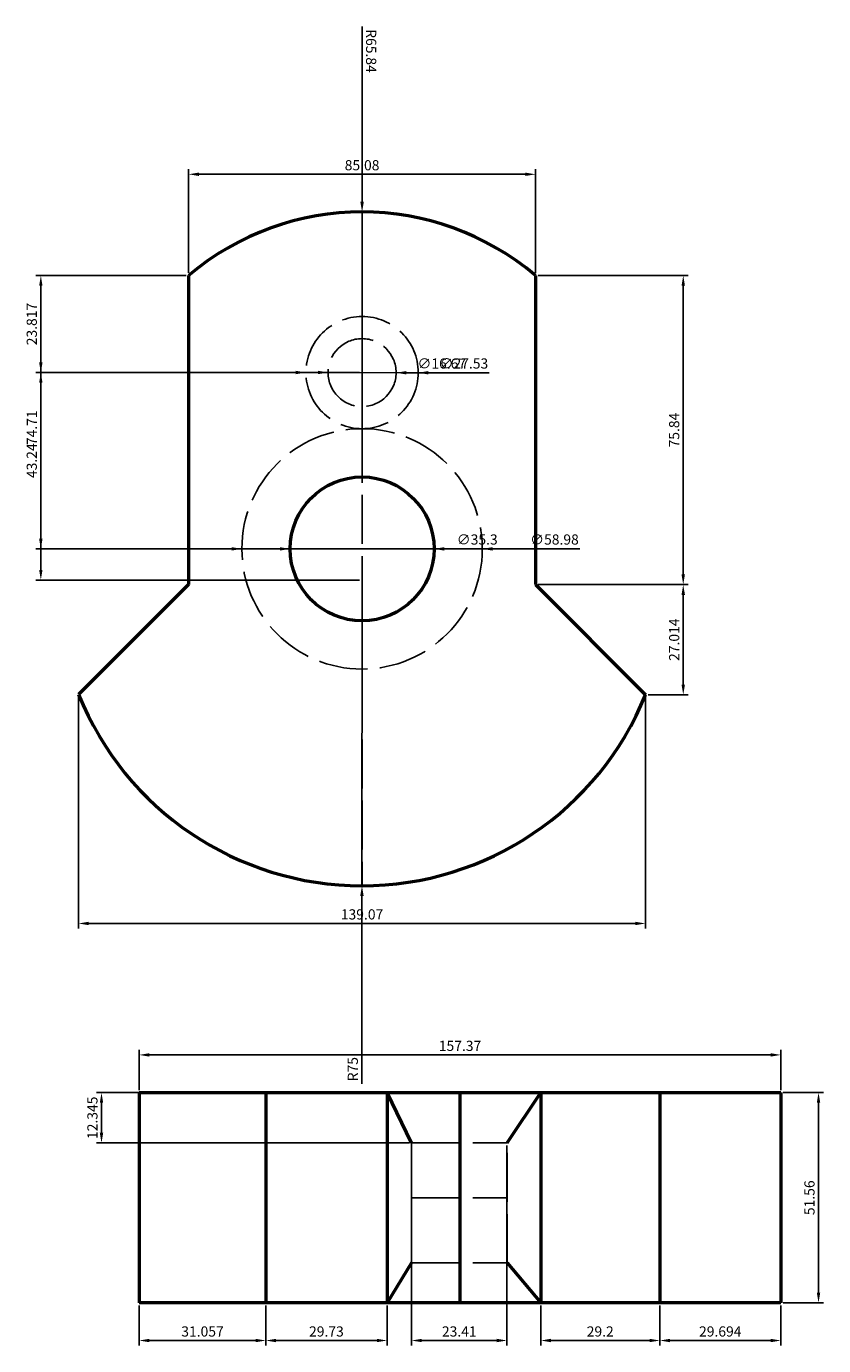
# Model space of a CAD drawing. Units: millimetres. Extents: x 921 to 2648, y 1390 to 2315.
# Tile 5 of 10: x 1425 to 1621, y 1915 to 2239. Entities that reach past the tile are written whole.
import ezdxf

# ---------------------------------------------------------------- set-up
doc = ezdxf.new("R2010")
doc.units = ezdxf.units.MM
doc.linetypes.add('ACAD_ISO02W100', pattern=[15, 12, -3])
for name, color, linetype, lineweight in [('M-DIMS', 2, 'Continuous', 25), ('M-HIDN', 4, 'ACAD_ISO02W100', 25), ('M-OUTL', 7, 'Continuous', 50)]:
    doc.layers.add(name, color=color, linetype=linetype, lineweight=lineweight)
doc.styles.get("Standard").update_dxf_attribs({"font": 'arial.ttf'})
doc.dimstyles.new('ISO-25', dxfattribs={"dimtxt": 2.5, "dimasz": 2.5, "dimexe": 1.25, "dimexo": 0.625, "dimtad": 1, "dimtxsty": 'Standard', "dimcen": 2.5, "dimadec": 0, "dimazin": 0, "dimtfac": 1, "dimtmove": 0, "dimatfit": 3, "dimfxl": 1, "dimarcsym": 0})

# ---------------------------------------------------------------- blocks, each defined once
blk = doc.blocks.new('*D26')
at = {"layer": 'Defpoints', "color": 0, "transparency": 16777216}
for p in [(1550.34, 2202.68), (1465.26, 2177.84), (1550.34, 2177.84)]:
    blk.add_point(p, dxfattribs=at)
at = {"layer": 'M-DIMS', "color": 0, "lineweight": -2, "transparency": 16777216}
for p, q in [((1465.26, 2178.47), (1465.26, 2203.93)), ((1467.76, 2202.68), (1547.84, 2202.68)), ((1550.34, 2178.47), (1550.34, 2203.93))]:
    blk.add_line(p, q, dxfattribs=at)
at = {"layer": 'M-DIMS', "color": 0, "transparency": 16777216}
for points in [[(1467.76, 2203.1), (1467.76, 2202.27), (1465.26, 2202.68)], [(1547.84, 2203.1), (1547.84, 2202.27), (1550.34, 2202.68)]]:
    blk.add_solid(points, dxfattribs=at)
at = {"layer": 'M-DIMS', "color": 0, "transparency": 16777216, "insert": (1507.8, 2204.58), "char_height": 2.5, "attachment_point": 5}
blk.add_mtext('85.08', dxfattribs=at)
blk = doc.blocks.new('*D27')
at = {"layer": 'Defpoints', "color": 0, "transparency": 16777216}
for p in [(1610.5, 1986.64), (1453.13, 1977.39), (1610.5, 1977.39)]:
    blk.add_point(p, dxfattribs=at)
at = {"layer": 'M-DIMS', "color": 0, "lineweight": -2, "transparency": 16777216}
for p, q in [((1453.13, 1978.01), (1453.13, 1987.89)), ((1610.5, 1978.01), (1610.5, 1987.89)), ((1455.63, 1986.64), (1608, 1986.64))]:
    blk.add_line(p, q, dxfattribs=at)
at = {"layer": 'M-DIMS', "color": 0, "transparency": 16777216}
for points in [[(1455.63, 1987.05), (1455.63, 1986.22), (1453.13, 1986.64)], [(1608, 1987.05), (1608, 1986.22), (1610.5, 1986.64)]]:
    blk.add_solid(points, dxfattribs=at)
at = {"layer": 'M-DIMS', "color": 0, "transparency": 16777216, "insert": (1531.82, 1988.54), "char_height": 2.5, "attachment_point": 5}
blk.add_mtext('157.37', dxfattribs=at)
blk = doc.blocks.new('*D28')
at = {"layer": 'Defpoints', "color": 0, "transparency": 16777216}
for p in [(1610.5, 1977.39), (1610.5, 1925.82), (1619.75, 1925.82)]:
    blk.add_point(p, dxfattribs=at)
at = {"layer": 'M-DIMS', "color": 0, "lineweight": -2, "transparency": 16777216}
for p, q in [((1611.12, 1977.39), (1621, 1977.39)), ((1619.75, 1974.89), (1619.75, 1928.32)), ((1611.12, 1925.82), (1621, 1925.82))]:
    blk.add_line(p, q, dxfattribs=at)
at = {"layer": 'M-DIMS', "color": 0, "transparency": 16777216}
for points in [[(1619.33, 1974.89), (1620.17, 1974.89), (1619.75, 1977.39)], [(1619.33, 1928.32), (1620.17, 1928.32), (1619.75, 1925.82)]]:
    blk.add_solid(points, dxfattribs=at)
at = {"layer": 'M-DIMS', "color": 0, "transparency": 16777216, "insert": (1617.85, 1951.6), "char_height": 2.5, "attachment_point": 5, "rotation": 90}
blk.add_mtext('51.56', dxfattribs=at)
blk = doc.blocks.new('*D62')
at = {"layer": 'Defpoints', "color": 0, "transparency": 16777216}
for p in [(1550.34, 2177.84), (1550.34, 2102.01), (1586.57, 2102.01)]:
    blk.add_point(p, dxfattribs=at)
at = {"layer": 'M-DIMS', "color": 0, "lineweight": -2, "transparency": 16777216}
for p, q in [((1550.96, 2177.84), (1587.82, 2177.84)), ((1586.57, 2175.34), (1586.57, 2104.51)), ((1550.96, 2102.01), (1587.82, 2102.01))]:
    blk.add_line(p, q, dxfattribs=at)
at = {"layer": 'M-DIMS', "color": 0, "transparency": 16777216}
for points in [[(1586.15, 2175.34), (1586.99, 2175.34), (1586.57, 2177.84)], [(1586.15, 2104.51), (1586.99, 2104.51), (1586.57, 2102.01)]]:
    blk.add_solid(points, dxfattribs=at)
at = {"layer": 'M-DIMS', "color": 0, "transparency": 16777216, "insert": (1584.67, 2139.93), "char_height": 2.5, "attachment_point": 5, "rotation": 90}
blk.add_mtext('75.84', dxfattribs=at)
blk = doc.blocks.new('*D63')
at = {"layer": 'Defpoints', "color": 0, "transparency": 16777216}
for p in [(1465.26, 2177.84), (1429.01, 2154.03), (1507.8, 2154.03)]:
    blk.add_point(p, dxfattribs=at)
at = {"layer": 'M-DIMS', "color": 0, "lineweight": -2, "transparency": 16777216}
for p, q in [((1464.64, 2177.84), (1427.76, 2177.84)), ((1429.01, 2175.34), (1429.01, 2156.53)), ((1507.18, 2154.03), (1427.76, 2154.03))]:
    blk.add_line(p, q, dxfattribs=at)
at = {"layer": 'M-DIMS', "color": 0, "transparency": 16777216}
for points in [[(1428.59, 2175.34), (1429.42, 2175.34), (1429.01, 2177.84)], [(1428.59, 2156.53), (1429.42, 2156.53), (1429.01, 2154.03)]]:
    blk.add_solid(points, dxfattribs=at)
at = {"layer": 'M-DIMS', "color": 0, "transparency": 16777216, "insert": (1427.1, 2165.94), "char_height": 2.5, "attachment_point": 5, "rotation": 90}
blk.add_mtext('23.817', dxfattribs=at)
blk = doc.blocks.new('*D64')
at = {"layer": 'Defpoints', "color": 0, "transparency": 16777216}
for p in [(1507.8, 2154.03), (1429.01, 2110.78), (1507.8, 2110.78)]:
    blk.add_point(p, dxfattribs=at)
at = {"layer": 'M-DIMS', "color": 0, "lineweight": -2, "transparency": 16777216}
for p, q in [((1507.18, 2154.03), (1427.76, 2154.03)), ((1429.01, 2151.53), (1429.01, 2113.28)), ((1507.18, 2110.78), (1427.76, 2110.78))]:
    blk.add_line(p, q, dxfattribs=at)
at = {"layer": 'M-DIMS', "color": 0, "transparency": 16777216}
for points in [[(1428.59, 2151.53), (1429.42, 2151.53), (1429.01, 2154.03)], [(1428.59, 2113.28), (1429.42, 2113.28), (1429.01, 2110.78)]]:
    blk.add_solid(points, dxfattribs=at)
at = {"layer": 'M-DIMS', "color": 0, "transparency": 16777216, "insert": (1427.1, 2132.41), "char_height": 2.5, "attachment_point": 5, "rotation": 90}
blk.add_mtext('43.24', dxfattribs=at)
blk = doc.blocks.new('*D65')
at = {"layer": 'Defpoints', "color": 0, "transparency": 16777216}
for p in [(1465.26, 2177.84), (1429.01, 2103.14), (1507.8, 2103.14)]:
    blk.add_point(p, dxfattribs=at)
at = {"layer": 'M-DIMS', "color": 0, "lineweight": -2, "transparency": 16777216}
for p, q in [((1464.64, 2177.84), (1427.76, 2177.84)), ((1429.01, 2175.34), (1429.01, 2105.64)), ((1507.18, 2103.14), (1427.76, 2103.14))]:
    blk.add_line(p, q, dxfattribs=at)
at = {"layer": 'M-DIMS', "color": 0, "transparency": 16777216}
for points in [[(1428.59, 2175.34), (1429.42, 2175.34), (1429.01, 2177.84)], [(1428.59, 2105.64), (1429.42, 2105.64), (1429.01, 2103.14)]]:
    blk.add_solid(points, dxfattribs=at)
at = {"layer": 'M-DIMS', "color": 0, "transparency": 16777216, "insert": (1427.13, 2140.49), "char_height": 2.5, "attachment_point": 5, "rotation": 90}
blk.add_mtext('74.71', dxfattribs=at)
blk = doc.blocks.new('*D66')
at = {"layer": 'Defpoints', "color": 0, "transparency": 16777216}
for p in [(1438.26, 2075.06), (1577.32, 2074.99), (1577.32, 2018.89)]:
    blk.add_point(p, dxfattribs=at)
at = {"layer": 'M-DIMS', "color": 0, "lineweight": -2, "transparency": 16777216}
for p, q in [((1438.26, 2074.43), (1438.26, 2017.64)), ((1577.32, 2074.37), (1577.32, 2017.64)), ((1440.76, 2018.89), (1574.82, 2018.89))]:
    blk.add_line(p, q, dxfattribs=at)
at = {"layer": 'M-DIMS', "color": 0, "transparency": 16777216}
for points in [[(1440.76, 2019.3), (1440.76, 2018.47), (1438.26, 2018.89)], [(1574.82, 2019.3), (1574.82, 2018.47), (1577.32, 2018.89)]]:
    blk.add_solid(points, dxfattribs=at)
at = {"layer": 'M-DIMS', "color": 0, "transparency": 16777216, "insert": (1507.79, 2020.79), "char_height": 2.5, "attachment_point": 5}
blk.add_mtext('139.07', dxfattribs=at)
blk = doc.blocks.new('*D67')
at = {"layer": 'Defpoints', "color": 0, "transparency": 16777216}
for p in [(1550.34, 2102.01), (1577.32, 2074.99), (1586.57, 2074.99)]:
    blk.add_point(p, dxfattribs=at)
at = {"layer": 'M-DIMS', "color": 0, "lineweight": -2, "transparency": 16777216}
for p, q in [((1550.96, 2102.01), (1587.82, 2102.01)), ((1586.57, 2099.51), (1586.57, 2077.49)), ((1577.95, 2074.99), (1587.82, 2074.99))]:
    blk.add_line(p, q, dxfattribs=at)
at = {"layer": 'M-DIMS', "color": 0, "transparency": 16777216}
for points in [[(1586.15, 2099.51), (1586.99, 2099.51), (1586.57, 2102.01)], [(1586.15, 2077.49), (1586.99, 2077.49), (1586.57, 2074.99)]]:
    blk.add_solid(points, dxfattribs=at)
at = {"layer": 'M-DIMS', "color": 0, "transparency": 16777216, "insert": (1584.67, 2088.5), "char_height": 2.5, "attachment_point": 5, "rotation": 90}
blk.add_mtext('27.014', dxfattribs=at)
blk = doc.blocks.new('*D68')
at = {"layer": 'Defpoints', "color": 0, "transparency": 16777216}
for p in [(1453.13, 1925.82), (1484.19, 1925.82), (1484.19, 1916.57)]:
    blk.add_point(p, dxfattribs=at)
at = {"layer": 'M-DIMS', "color": 0, "lineweight": -2, "transparency": 16777216}
for p, q in [((1453.13, 1925.2), (1453.13, 1915.32)), ((1484.19, 1925.2), (1484.19, 1915.32)), ((1455.63, 1916.57), (1481.69, 1916.57))]:
    blk.add_line(p, q, dxfattribs=at)
at = {"layer": 'M-DIMS', "color": 0, "transparency": 16777216}
for points in [[(1455.63, 1916.99), (1455.63, 1916.16), (1453.13, 1916.57)], [(1481.69, 1916.99), (1481.69, 1916.16), (1484.19, 1916.57)]]:
    blk.add_solid(points, dxfattribs=at)
at = {"layer": 'M-DIMS', "color": 0, "transparency": 16777216, "insert": (1468.66, 1918.47), "char_height": 2.5, "attachment_point": 5}
blk.add_mtext('31.057', dxfattribs=at)
blk = doc.blocks.new('*D69')
at = {"layer": 'Defpoints', "color": 0, "transparency": 16777216}
for p in [(1484.19, 1925.82), (1513.92, 1925.82), (1513.92, 1916.57)]:
    blk.add_point(p, dxfattribs=at)
at = {"layer": 'M-DIMS', "color": 0, "lineweight": -2, "transparency": 16777216}
for p, q in [((1484.19, 1925.2), (1484.19, 1915.32)), ((1513.92, 1925.2), (1513.92, 1915.32)), ((1486.69, 1916.57), (1511.42, 1916.57))]:
    blk.add_line(p, q, dxfattribs=at)
at = {"layer": 'M-DIMS', "color": 0, "transparency": 16777216}
for points in [[(1486.69, 1916.99), (1486.69, 1916.16), (1484.19, 1916.57)], [(1511.42, 1916.99), (1511.42, 1916.16), (1513.92, 1916.57)]]:
    blk.add_solid(points, dxfattribs=at)
at = {"layer": 'M-DIMS', "color": 0, "transparency": 16777216, "insert": (1499.05, 1918.47), "char_height": 2.5, "attachment_point": 5}
blk.add_mtext('29.73', dxfattribs=at)
blk = doc.blocks.new('*D70')
at = {"layer": 'Defpoints', "color": 0, "transparency": 16777216}
for p in [(1551.61, 1925.82), (1580.81, 1925.82), (1580.81, 1916.57)]:
    blk.add_point(p, dxfattribs=at)
at = {"layer": 'M-DIMS', "color": 0, "lineweight": -2, "transparency": 16777216}
for p, q in [((1551.61, 1925.2), (1551.61, 1915.32)), ((1580.81, 1925.2), (1580.81, 1915.32)), ((1554.11, 1916.57), (1578.31, 1916.57))]:
    blk.add_line(p, q, dxfattribs=at)
at = {"layer": 'M-DIMS', "color": 0, "transparency": 16777216}
for points in [[(1554.11, 1916.99), (1554.11, 1916.16), (1551.61, 1916.57)], [(1578.31, 1916.99), (1578.31, 1916.16), (1580.81, 1916.57)]]:
    blk.add_solid(points, dxfattribs=at)
at = {"layer": 'M-DIMS', "color": 0, "transparency": 16777216, "insert": (1566.21, 1918.47), "char_height": 2.5, "attachment_point": 5}
blk.add_mtext('29.2', dxfattribs=at)
blk = doc.blocks.new('*D71')
at = {"layer": 'Defpoints', "color": 0, "transparency": 16777216}
for p in [(1580.81, 1925.82), (1610.5, 1925.82), (1610.5, 1916.57)]:
    blk.add_point(p, dxfattribs=at)
at = {"layer": 'M-DIMS', "color": 0, "lineweight": -2, "transparency": 16777216}
for p, q in [((1580.81, 1925.2), (1580.81, 1915.32)), ((1610.5, 1925.2), (1610.5, 1915.32)), ((1583.31, 1916.57), (1608, 1916.57))]:
    blk.add_line(p, q, dxfattribs=at)
at = {"layer": 'M-DIMS', "color": 0, "transparency": 16777216}
for points in [[(1583.31, 1916.99), (1583.31, 1916.16), (1580.81, 1916.57)], [(1608, 1916.99), (1608, 1916.16), (1610.5, 1916.57)]]:
    blk.add_solid(points, dxfattribs=at)
at = {"layer": 'M-DIMS', "color": 0, "transparency": 16777216, "insert": (1595.65, 1918.47), "char_height": 2.5, "attachment_point": 5}
blk.add_mtext('29.694', dxfattribs=at)
blk = doc.blocks.new('*D72')
at = {"layer": 'Defpoints', "color": 0, "transparency": 16777216}
for p in [(1519.94, 1965.04), (1543.34, 1965.04), (1543.34, 1916.57)]:
    blk.add_point(p, dxfattribs=at)
at = {"layer": 'M-DIMS', "color": 0, "lineweight": -2, "transparency": 16777216}
for p, q in [((1519.94, 1964.42), (1519.94, 1915.32)), ((1543.34, 1964.42), (1543.34, 1915.32)), ((1522.44, 1916.57), (1540.84, 1916.57))]:
    blk.add_line(p, q, dxfattribs=at)
at = {"layer": 'M-DIMS', "color": 0, "transparency": 16777216}
for points in [[(1522.44, 1916.99), (1522.44, 1916.16), (1519.94, 1916.57)], [(1540.84, 1916.99), (1540.84, 1916.16), (1543.34, 1916.57)]]:
    blk.add_solid(points, dxfattribs=at)
at = {"layer": 'M-DIMS', "color": 0, "transparency": 16777216, "insert": (1531.64, 1918.47), "char_height": 2.5, "attachment_point": 5}
blk.add_mtext('23.41', dxfattribs=at)
blk = doc.blocks.new('*D73')
at = {"layer": 'Defpoints', "color": 0, "transparency": 16777216}
for p in [(1513.92, 1977.39), (1443.88, 1965.04), (1519.94, 1965.04)]:
    blk.add_point(p, dxfattribs=at)
at = {"layer": 'M-DIMS', "color": 0, "lineweight": -2, "transparency": 16777216}
for p, q in [((1513.29, 1977.39), (1442.63, 1977.39)), ((1443.88, 1974.89), (1443.88, 1967.54)), ((1519.31, 1965.04), (1442.63, 1965.04))]:
    blk.add_line(p, q, dxfattribs=at)
at = {"layer": 'M-DIMS', "color": 0, "transparency": 16777216}
for points in [[(1443.47, 1974.89), (1444.3, 1974.89), (1443.88, 1977.39)], [(1443.47, 1967.54), (1444.3, 1967.54), (1443.88, 1965.04)]]:
    blk.add_solid(points, dxfattribs=at)
at = {"layer": 'M-DIMS', "color": 0, "transparency": 16777216, "insert": (1441.98, 1971.21), "char_height": 2.5, "attachment_point": 5, "rotation": 90}
blk.add_mtext('12.345', dxfattribs=at)
blk = doc.blocks.new('*D110')
at = {"layer": 'Defpoints', "color": 0, "transparency": 16777216}
for p in [(1507.8, 2103.14), (1507.77, 2028.14)]:
    blk.add_point(p, dxfattribs=at)
at = {"layer": 'M-DIMS', "color": 0, "lineweight": -2, "transparency": 16777216}
for p, q in [((1507.8, 2103.14), (1507.77, 2028.14)), ((1507.75, 1979.51), (1507.77, 2025.64))]:
    blk.add_line(p, q, dxfattribs=at)
at = {"layer": 'M-DIMS', "color": 0, "transparency": 16777216}
blk.add_solid([(1507.35, 2025.64), (1508.18, 2025.64), (1507.77, 2028.14)], dxfattribs=at)
at = {"layer": 'M-DIMS', "color": 0, "transparency": 16777216, "insert": (1505.85, 1983.14), "char_height": 2.5, "attachment_point": 5, "rotation": 89.9746}
blk.add_mtext('R75', dxfattribs=at)
blk = doc.blocks.new('*D111')
at = {"layer": 'Defpoints', "color": 0, "transparency": 16777216}
for p in [(1507.8, 2193.43), (1507.8, 2127.6)]:
    blk.add_point(p, dxfattribs=at)
at = {"layer": 'M-DIMS', "color": 0, "lineweight": -2, "transparency": 16777216}
for p, q in [((1507.8, 2238.97), (1507.8, 2195.93)), ((1507.8, 2127.6), (1507.8, 2193.43))]:
    blk.add_line(p, q, dxfattribs=at)
at = {"layer": 'M-DIMS', "color": 0, "transparency": 16777216}
blk.add_solid([(1508.22, 2195.93), (1507.38, 2195.93), (1507.8, 2193.43)], dxfattribs=at)
at = {"layer": 'M-DIMS', "color": 0, "transparency": 16777216, "insert": (1509.7, 2232.93), "char_height": 2.5, "attachment_point": 5, "rotation": 270.0002}
blk.add_mtext('R65.84', dxfattribs=at)
blk = doc.blocks.new('*D112')
at = {"layer": 'Defpoints', "color": 0, "transparency": 16777216}
for p in [(1478.31, 2110.78), (1537.29, 2110.78)]:
    blk.add_point(p, dxfattribs=at)
at = {"layer": 'M-DIMS', "color": 0, "lineweight": -2, "transparency": 16777216}
for p, q in [((1475.81, 2110.78), (1473.31, 2110.78)), ((1478.31, 2110.78), (1537.29, 2110.78)), ((1561.19, 2110.78), (1539.79, 2110.78))]:
    blk.add_line(p, q, dxfattribs=at)
at = {"layer": 'M-DIMS', "color": 0, "transparency": 16777216}
for points in [[(1475.81, 2111.2), (1475.81, 2110.37), (1478.31, 2110.78)], [(1539.79, 2111.2), (1539.79, 2110.37), (1537.29, 2110.78)]]:
    blk.add_solid(points, dxfattribs=at)
at = {"layer": 'M-DIMS', "color": 0, "transparency": 16777216, "insert": (1554.99, 2112.76), "char_height": 2.5, "attachment_point": 5, "rotation": 0.0003}
blk.add_mtext('∅58.98', dxfattribs=at)
blk = doc.blocks.new('*D113')
at = {"layer": 'Defpoints', "color": 0, "transparency": 16777216}
for p in [(1490.15, 2110.78), (1525.45, 2110.78)]:
    blk.add_point(p, dxfattribs=at)
at = {"layer": 'M-DIMS', "color": 0, "lineweight": -2, "transparency": 16777216}
for p, q in [((1487.65, 2110.78), (1485.15, 2110.78)), ((1490.15, 2110.78), (1525.45, 2110.78)), ((1541.27, 2110.78), (1527.95, 2110.78))]:
    blk.add_line(p, q, dxfattribs=at)
at = {"layer": 'M-DIMS', "color": 0, "transparency": 16777216}
for points in [[(1487.65, 2111.2), (1487.65, 2110.37), (1490.15, 2110.78)], [(1527.95, 2111.2), (1527.95, 2110.37), (1525.45, 2110.78)]]:
    blk.add_solid(points, dxfattribs=at)
at = {"layer": 'M-DIMS', "color": 0, "transparency": 16777216, "insert": (1536.04, 2112.76), "char_height": 2.5, "attachment_point": 5, "rotation": 0.0005}
blk.add_mtext('∅35.3', dxfattribs=at)
blk = doc.blocks.new('*D134')
at = {"layer": 'Defpoints', "color": 0, "transparency": 16777216}
for p in [(1494.04, 2154.05), (1521.57, 2154)]:
    blk.add_point(p, dxfattribs=at)
at = {"layer": 'M-DIMS', "color": 0, "lineweight": -2, "transparency": 16777216}
for p, q in [((1491.54, 2154.06), (1489.04, 2154.06)), ((1494.04, 2154.05), (1521.57, 2154)), ((1538.97, 2153.97), (1524.07, 2153.99))]:
    blk.add_line(p, q, dxfattribs=at)
at = {"layer": 'M-DIMS', "color": 0, "transparency": 16777216}
for points in [[(1491.54, 2154.48), (1491.54, 2153.64), (1494.04, 2154.05)], [(1524.07, 2154.41), (1524.07, 2153.58), (1521.57, 2154)]]:
    blk.add_solid(points, dxfattribs=at)
at = {"layer": 'M-DIMS', "color": 0, "transparency": 16777216, "insert": (1532.77, 2155.95), "char_height": 2.5, "attachment_point": 5, "rotation": 359.887}
blk.add_mtext('∅27.53', dxfattribs=at)
blk = doc.blocks.new('*D135')
at = {"layer": 'Defpoints', "color": 0, "transparency": 16777216}
for p in [(1499.47, 2154.05), (1516.14, 2154)]:
    blk.add_point(p, dxfattribs=at)
at = {"layer": 'M-DIMS', "color": 0, "lineweight": -2, "transparency": 16777216}
for p, q in [((1496.97, 2154.06), (1494.47, 2154.07)), ((1499.47, 2154.05), (1516.14, 2154)), ((1533.54, 2153.94), (1518.64, 2153.99))]:
    blk.add_line(p, q, dxfattribs=at)
at = {"layer": 'M-DIMS', "color": 0, "transparency": 16777216}
for points in [[(1496.97, 2154.48), (1496.97, 2153.65), (1499.47, 2154.05)], [(1518.64, 2154.41), (1518.63, 2153.58), (1516.14, 2154)]]:
    blk.add_solid(points, dxfattribs=at)
at = {"layer": 'M-DIMS', "color": 0, "transparency": 16777216, "insert": (1527.35, 2155.93), "char_height": 2.5, "attachment_point": 5, "rotation": 359.8135}
blk.add_mtext('∅16.67', dxfattribs=at)

msp = doc.modelspace()

# ---------------------------------------------------------------- linework, layer by layer
at = {"layer": 'M-HIDN'}
for p, q in [((1507.8013, 2154.027), (1507.8013, 2028.1356)), ((1519.9364, 1965.0415), (1543.3441, 1965.0415)), ((1519.9364, 1965.0415), (1519.9364, 1935.5986)), ((1543.3441, 1935.5986), (1543.3441, 1965.0415)), ((1519.9364, 1951.6042), (1543.3441, 1951.6042)), ((1519.9364, 1935.5986), (1543.3441, 1935.5986))]:
    msp.add_line(p, q, dxfattribs=at)
for centre, radius in [((1507.8013, 2154.027), 13.7647), ((1507.8013, 2154.027), 8.3349), ((1507.8013, 2110.7838), 29.4918)]:
    msp.add_circle(centre, radius, dxfattribs=at)
at = {"layer": 'M-OUTL'}
for p, q in [((1465.2628, 2177.8438), (1465.2628, 2102.0083)), ((1550.3397, 2177.8438), (1550.3397, 2102.0083)), ((1465.2628, 2102.0083), (1438.2559, 2075.0563)), ((1550.3397, 2102.0083), (1577.3216, 2074.9943)), ((1453.1322, 1977.3865), (1610.4997, 1977.3865)), ((1453.1322, 1977.3865), (1453.1322, 1925.8219)), ((1484.1888, 1977.3865), (1484.1888, 1925.8219)), ((1513.9171, 1977.3865), (1513.9171, 1925.8219)), ((1519.9364, 1965.0415), (1513.9171, 1977.3865)), ((1531.8159, 1977.3865), (1531.8159, 1925.8219)), ((1543.3441, 1965.0415), (1551.6083, 1977.3865)), ((1551.6083, 1977.3865), (1551.6083, 1925.8219)), ((1580.8058, 1977.3865), (1580.8058, 1925.8219)), ((1610.4997, 1977.3865), (1610.4997, 1925.8219)), ((1519.9364, 1935.5986), (1513.9171, 1925.8219)), ((1543.3441, 1935.5986), (1551.6083, 1925.8219)), ((1610.4997, 1925.8219), (1453.1322, 1925.8219))]:
    msp.add_line(p, q, dxfattribs=at)
msp.add_circle((1507.8013, 2110.7838), 17.6506, dxfattribs=at)
for centre, radius, start, end in [((1507.8013, 2127.5969), 65.8352, 49.74918, 130.25082), ((1507.8013, 2103.1356), 75, 201.986599, 337.962253)]:
    msp.add_arc(centre, radius, start, end, dxfattribs=at)

# ---------------------------------------------------------------- dimensions: what is measured, and where the dimension line sits
at = {"layer": 'M-DIMS'}
for center, mpoint, override, picture, middle in [((1507.8013, 2127.5969), (1507.801, 2193.4321), {"dimdec": 2, "dimlfac": 1, "dimrnd": 0, "dimzin": 0, "dimdsep": 46, "dimlunit": 2}, '*D111', (1507.8008, 2232.9332)), ((1507.8013, 2103.1356), (1507.768, 2028.1356), {"dimdec": 0, "dimlfac": 1, "dimrnd": 0, "dimzin": 0, "dimdsep": 46, "dimlunit": 2}, '*D110', (1507.748, 1983.1356))]:
    dim = msp.add_radius_dim(center=center, mpoint=mpoint, dimstyle='ISO-25', override=override, dxfattribs=at)
    dim.commit()
    dim.dimension.update_dxf_attribs({"geometry": picture, "text_midpoint": middle, "dimtype": 164})
for base, p1, p2, override, picture, middle in [((1550.3397, 2202.6821), (1465.2628, 2177.8438), (1550.3397, 2177.8438), {"dimdec": 2, "dimlfac": 1, "dimrnd": 0, "dimzin": 0, "dimdsep": 46, "dimlunit": 2}, '*D26', (1507.8013, 2204.5835)), ((1577.3216, 2018.8856), (1438.2559, 2075.0563), (1577.3216, 2074.9943), {"dimdec": 2, "dimlfac": 1, "dimrnd": 0, "dimzin": 0, "dimdsep": 46, "dimlunit": 2}, '*D66', (1507.7887, 2020.7879)), ((1610.4997, 1986.6365), (1453.1322, 1977.3865), (1610.4997, 1977.3865), {"dimdec": 2, "dimlfac": 1, "dimrnd": 0, "dimzin": 0, "dimdsep": 46, "dimlunit": 2}, '*D27', (1531.8159, 1988.5388)), ((1543.3441, 1916.5719), (1519.9364, 1965.0415), (1543.3441, 1965.0415), {"dimdec": 2, "dimlfac": 1, "dimrnd": 0, "dimzin": 0, "dimdsep": 46, "dimlunit": 2}, '*D72', (1531.6402, 1918.4742)), ((1484.1888, 1916.5719), (1453.1322, 1925.8219), (1484.1888, 1925.8219), {"dimdec": 3, "dimlfac": 1, "dimrnd": 0, "dimzin": 0, "dimdsep": 46, "dimlunit": 2}, '*D68', (1468.6605, 1918.4742)), ((1513.9171, 1916.5719), (1484.1888, 1925.8219), (1513.9171, 1925.8219), {"dimdec": 2, "dimlfac": 1, "dimrnd": 0, "dimzin": 0, "dimdsep": 46, "dimlunit": 2}, '*D69', (1499.0529, 1918.4742)), ((1580.8058, 1916.5719), (1551.6083, 1925.8219), (1580.8058, 1925.8219), {"dimdec": 1, "dimlfac": 1, "dimrnd": 0, "dimzin": 0, "dimdsep": 46, "dimlunit": 2}, '*D70', (1566.207, 1918.4733)), ((1610.4997, 1916.5719), (1580.8058, 1925.8219), (1610.4997, 1925.8219), {"dimdec": 3, "dimlfac": 1, "dimrnd": 0, "dimzin": 0, "dimdsep": 46, "dimlunit": 2}, '*D71', (1595.6527, 1918.4733))]:
    dim = msp.add_linear_dim(base=base, p1=p1, p2=p2, dimstyle='ISO-25', override=override, dxfattribs=at)
    dim.commit()
    dim.dimension.update_dxf_attribs({"geometry": picture, "text_midpoint": middle})
for base, p1, p2, override, picture, middle in [((1429.0059, 2154.027), (1465.2628, 2177.8438), (1507.8013, 2154.027), {"dimdec": 3, "dimlfac": 1, "dimrnd": 0, "dimzin": 0, "dimdsep": 46, "dimlunit": 2}, '*D63', (1427.1036, 2165.9354)), ((1429.0059, 2103.1356), (1465.2628, 2177.8438), (1507.8013, 2103.1356), {"dimdec": 2, "dimlfac": 1, "dimrnd": 0, "dimzin": 0, "dimdsep": 46, "dimlunit": 2}, '*D65', (1427.1258, 2140.4897)), ((1586.5716, 2102.0083), (1550.3397, 2177.8438), (1550.3397, 2102.0083), {"dimdec": 2, "dimlfac": 1, "dimrnd": 0, "dimzin": 0, "dimdsep": 46, "dimlunit": 2}, '*D62', (1584.6701, 2139.9261)), ((1429.0059, 2110.7838), (1507.8013, 2154.027), (1507.8013, 2110.7838), {"dimdec": 2, "dimlfac": 1, "dimrnd": 0, "dimzin": 0, "dimdsep": 46, "dimlunit": 2}, '*D64', (1427.1036, 2132.4054)), ((1586.5716, 2074.9943), (1550.3397, 2102.0083), (1577.3216, 2074.9943), {"dimdec": 3, "dimlfac": 1, "dimrnd": 0, "dimzin": 0, "dimdsep": 46, "dimlunit": 2}, '*D67', (1584.6701, 2088.5013)), ((1443.8822, 1965.0415), (1513.9171, 1977.3865), (1519.9364, 1965.0415), {"dimdec": 3, "dimlfac": 1, "dimrnd": 0, "dimzin": 0, "dimdsep": 46, "dimlunit": 2}, '*D73', (1441.9799, 1971.214)), ((1619.7497, 1925.8219), (1610.4997, 1977.3865), (1610.4997, 1925.8219), {"dimdec": 2, "dimlfac": 1, "dimrnd": 0, "dimzin": 0, "dimdsep": 46, "dimlunit": 2}, '*D28', (1617.8482, 1951.6042))]:
    dim = msp.add_linear_dim(base=base, p1=p1, p2=p2, angle=90, dimstyle='ISO-25', override=override, dxfattribs=at)
    dim.commit()
    dim.dimension.update_dxf_attribs({"geometry": picture, "text_midpoint": middle})
for p1, p2, override, picture, middle in [((1494.0366, 2154.0542), (1521.566, 2153.9999), {"dimdec": 2, "dimlfac": 1, "dimrnd": 0, "dimzin": 0, "dimdsep": 46, "dimlunit": 2}, '*D134', (1532.769, 2153.9778)), ((1499.4664, 2154.0541), (1516.1362, 2153.9999), {"dimdec": 2, "dimlfac": 1, "dimrnd": 0, "dimzin": 0, "dimdsep": 46, "dimlunit": 2}, '*D135', (1527.3392, 2153.9634)), ((1478.3095, 2110.7837), (1537.2931, 2110.784), {"dimdec": 2, "dimlfac": 1, "dimrnd": 0, "dimzin": 0, "dimdsep": 46, "dimlunit": 2}, '*D112', (1554.9882, 2110.7841)), ((1490.1507, 2110.7837), (1525.4519, 2110.784), {"dimdec": 1, "dimlfac": 1, "dimrnd": 0, "dimzin": 0, "dimdsep": 46, "dimlunit": 2}, '*D113', (1536.0422, 2110.7841))]:
    dim = msp.add_diameter_dim_2p(p1=p1, p2=p2, dimstyle='ISO-25', override=override, dxfattribs=at)
    dim.commit()
    dim.dimension.update_dxf_attribs({"geometry": picture, "text_midpoint": middle, "dimtype": 163})

doc.saveas('drawing.dxf')
